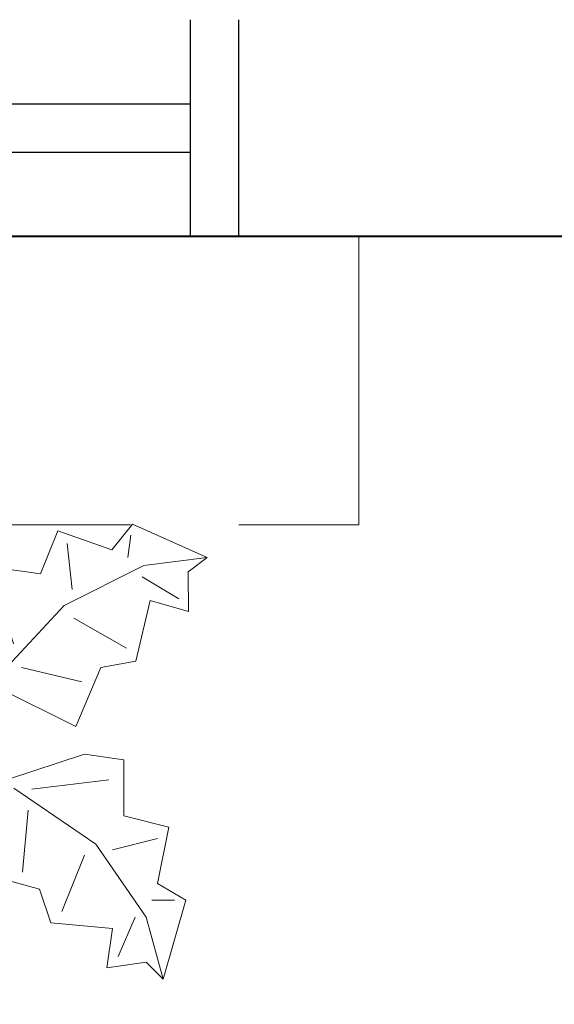
# Model space of a CAD drawing. Units: inches. Extents: x -301 to 715, y -607 to 364.
# Tile 87 of 141: x 74 to 96, y -256 to -215. Entities that reach past the tile are written whole.
import ezdxf

# ---------------------------------------------------------------- set-up
doc = ezdxf.new("R2010")
doc.units = ezdxf.units.IN
doc.header["$MEASUREMENT"] = 0
doc.linetypes.add('ACAD_ISO02W100', pattern=[15, 12, -3])
for name, color, linetype, lineweight in [('A-GLAZ', 2, 'Continuous', 25), ('A-GLAZ-OVHD', 2, 'ACAD_ISO02W100', 18), ('A-WALL', 3, 'Continuous', 40), ('L-PLNT', 94, 'Continuous', 13)]:
    doc.layers.add(name, color=color, linetype=linetype, lineweight=lineweight)

# ---------------------------------------------------------------- blocks, each defined once
blk = doc.blocks.new('Plant - Rubber or Philodendron')
for p, q in [((13.3837, 12.301), (14.68, 13.9039)), ((14.68, 13.9039), (19.3848, 11.8146)), ((8.8871, 10.7908), (9.9809, 13.4933)), ((9.9809, 13.4933), (13.3837, 12.301)), ((14.5816, 13.2037), (14.3848, 11.8033)), ((10.5828, 12.6946), (10.8893, 9.7953)), ((-14.8639, 10.7964), (-12.6195, 11.8975)), ((-12.6195, 11.8975), (-12.1909, 9.4345)), ((19.3848, 11.8146), (15.3859, 11.3055)), ((19.3848, 11.8146), (18.1868, 10.9119)), ((-16.2005, 11.4774), (-13.9899, 8.1064)), ((-16.2005, 11.4774), (-14.8639, 10.7964)), ((-16.0159, 6.3329), (-16.2005, 11.4774)), ((4.6914, 8.8812), (5.3859, 11.2828)), ((5.3859, 11.2828), (8.8871, 10.7908)), ((15.3859, 11.3055), (10.3916, 8.7942)), ((-13.3174, 8.325), (-13.0735, 11.0065)), ((15.2875, 10.6053), (17.5907, 9.2105)), ((18.1868, 10.9119), (18.1925, 8.4119)), ((-12.1909, 9.4345), (-8.3829, 10.3)), ((-8.3829, 10.3), (-7.0549, 8.501)), ((5.9878, 10.4842), (7.1971, 6.3869)), ((-8.8369, 9.409), (-9.0894, 5.6095)), ((-7.0549, 8.501), (-3.0284, 8.6941)), ((-3.0284, 8.6941), (-3.0709, 3.1041)), ((4.6914, 8.8812), (5.5014, 4.4831)), ((10.3916, 8.7942), (6.2847, 4.4028)), ((15.7909, 9.1065), (14.8995, 5.3044)), ((18.1925, 8.4119), (15.7909, 9.1065)), ((-13.9899, 8.1064), (-9.5434, 4.7185)), ((-4.8529, 4.012), (-5.7184, 7.82)), ((14.2977, 6.1031), (10.9934, 7.9956)), ((-15.3434, 6.5514), (-13.9984, 6.9884)), ((-14.0069, 5.8704), (-16.0159, 6.3329)), ((-13.5868, 2.2894), (-14.0069, 5.8704)), ((14.8995, 5.3044), (12.7005, 4.8994)), ((-13.1329, 3.1804), (-10.6614, 4.727)), ((-9.5434, 4.7185), (-4.1917, 2.9888)), ((5.4346, 3.9146), (5.5014, 4.4831)), ((7.7005, 4.8881), (11.5025, 3.9967)), ((12.7005, 4.8994), (11.1089, 1.1958)), ((2.1141, 0.2298), (5.4346, 3.9146)), ((-3.0709, 3.1041), (0.0797, 2.3163)), ((6.1032, 3.6844), (2.8262, -0.031)), ((11.1089, 1.1958), (6.1032, 3.6844)), ((-10.6784, 2.491), (-13.5868, 2.2894)), ((-9.5858, -0.8715), (-10.6784, 2.491)), ((-9.1318, 0.0195), (-5.9793, 2.9025)), ((-7.1228, -0.443), (-3.5248, 2.2131)), ((-3.5248, 2.2131), (-3.3011, 2.4355)), ((-3.3011, 2.4355), (-0.5306, 1.7947)), ((0.0797, 2.3163), (0.4866, -0.031)), ((-0.5306, 1.7947), (-0.2255, -0.5527)), ((-0.5306, 1.7947), (-0.5306, 1.7947)), ((0.4866, -0.031), (2.1141, 0.2298)), ((-7.1228, -0.443), (-9.5858, -0.8715)), ((-2.019, -3.6148), (-0.2255, -0.5527)), ((2.8262, -0.031), (1.3003, -0.5527)), ((1.3003, -0.5527), (2.4193, -1.4655)), ((11.6605, -0.5413), (6.895, -2.1175)), ((11.6605, -0.5413), (14.1354, -0.8948)), ((-0.9375, -3.1608), (0.5883, -0.8135)), ((0.5883, -0.8135), (2.2447, -2.0916)), ((14.1354, -0.8948), (14.1354, -4.4304)), ((2.4193, -1.4655), (6.895, -2.1175)), ((2.2447, -2.0916), (6.7108, -2.6626)), ((8.3544, -2.7453), (13.1973, -2.1704)), ((4.943, -7.9659), (6.7108, -2.6626)), ((12.3677, -6.1981), (7.219, -2.6772)), ((-11.3237, -7.2629), (-9.7321, -3.5593)), ((-9.7321, -3.5593), (-4.7264, -6.0479)), ((-2.019, -3.6148), (-4.7264, -6.0479)), ((-4.0579, -6.2781), (-0.9375, -3.1608)), ((8.125, -4.0768), (7.7715, -7.9659)), ((14.1354, -4.4304), (16.9638, -5.1375)), ((16.9638, -5.1375), (16.2567, -8.673)), ((16.2567, -5.8446), (13.4283, -6.5517)), ((-6.3237, -7.2516), (-10.1257, -6.3602)), ((-4.1246, -6.8466), (-4.0579, -6.2781)), ((15.5496, -10.7943), (12.3677, -6.1981)), ((-13.5228, -7.6679), (-11.3237, -7.2629)), ((-9.0148, -11.1577), (-4.9047, -6.8122)), ((-3.3146, -11.2447), (-4.1246, -6.8466)), ((10.2463, -10.4408), (11.6605, -6.9053)), ((-14.4141, -11.4699), (-13.5228, -7.6679)), ((8.8321, -9.0266), (4.943, -7.9659)), ((-12.921, -8.4665), (-9.6166, -10.359)), ((-4.611, -12.8477), (-5.8203, -8.7504)), ((9.5392, -11.1479), (8.8321, -9.0266)), ((16.2567, -8.673), (18.0245, -9.7337)), ((17.3174, -9.7337), (15.9032, -9.7337)), ((18.0245, -9.7337), (16.6103, -14.6834)), ((-16.8157, -10.7754), (-14.4141, -11.4699)), ((-16.8101, -13.2754), (-16.8157, -10.7754)), ((14.8425, -10.7943), (13.7819, -13.2692)), ((16.6103, -14.6834), (15.5496, -10.7943)), ((-13.9107, -12.9688), (-16.2139, -11.574)), ((-14.0091, -13.669), (-9.0148, -11.1577)), ((-3.3146, -11.2447), (-4.0092, -13.6463)), ((13.4283, -11.5015), (9.5392, -11.1479)), ((13.0748, -13.9763), (13.4283, -11.5015)), ((-9.206, -15.0581), (-9.5126, -12.1588)), ((-18.008, -14.1781), (-16.8101, -13.2754)), ((-7.5103, -13.1543), (-8.6042, -15.8568)), ((-4.0092, -13.6463), (-7.5103, -13.1543)), ((-18.008, -14.1781), (-14.0091, -13.669)), ((-13.3032, -16.2674), (-18.008, -14.1781)), ((-13.2048, -15.5672), (-13.008, -14.1668)), ((15.5496, -13.6228), (13.0748, -13.9763)), ((16.6103, -14.6834), (15.5496, -13.6228)), ((-12.0069, -14.6645), (-13.3032, -16.2674)), ((-8.6042, -15.8568), (-12.0069, -14.6645))]:
    blk.add_line(p, q)
for centre, radius, start, end in [((0, 0), 6.1275, 34.37569, 120.1028), ((-0.0601, -0.2075), 5.2461, 33.82192, 124.9414), ((-0.098, 0.1364), 6.1288, 341.2017, 26.09184), ((-0.2664, 0.1682), 5.2775, 338.4094, 20.03007), ((0.0308, 0.1664), 5, 168.1647, 238.6725), ((0.0308, 0.1664), 6, 178.6147, 235.1169), ((-0.1102, 0.4886), 5.2883, 247.3711, 327.472), ((-0.0234, 0.3825), 6.1492, 242.5812, 331.2714)]:
    blk.add_arc(centre, radius, start, end)
blk = doc.blocks.new('WIN-36-PLAN')
for p, q in [((0, 0), (0, 9)), ((2, 0), (2, 9)), ((20, 0), (20, 9)), ((38, 0), (38, 9)), ((40, 0), (40, 9)), ((2, 5.5), (38, 5.5)), ((2, 3.5), (38, 3.5))]:
    blk.add_line(p, q)
blk = doc.blocks.new('WIN-SHADE-50')
at = {"ltscale": 1.5}
for p, q in [((0, 0), (0, 12)), ((50, 12), (0, 12)), ((50, 0), (50, 12)), ((5, 0), (0, 0)), ((45, 0), (50, 0))]:
    blk.add_line(p, q, dxfattribs=at)

msp = doc.modelspace()

# ---------------------------------------------------------------- linework, layer by layer
at = {"layer": 'A-WALL'}
msp.add_line((-45.603, -223.818), (132.897, -223.818), dxfattribs=at)

# ---------------------------------------------------------------- block references
at = {"layer": 'A-GLAZ'}
msp.add_blockref('WIN-36-PLAN', (43.147, -223.818), dxfattribs=at)
at = {"layer": 'A-GLAZ-OVHD', "rotation": 180}
msp.add_blockref('WIN-SHADE-50', (88.146, -223.817), dxfattribs=at)
at = {"layer": 'L-PLNT', "xscale": 0.6613521884636907, "yscale": 0.6613521884636907, "zscale": 0.6613521884636907}
msp.add_blockref('Plant - Rubber or Philodendron', (69.022, -244.98), dxfattribs=at)

doc.saveas('drawing.dxf')
